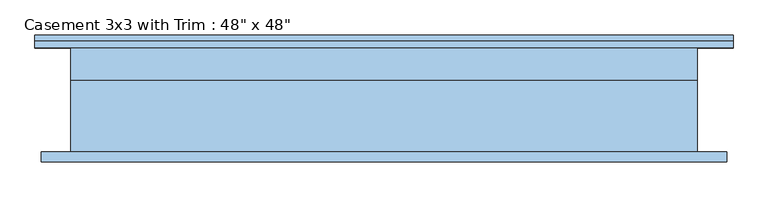
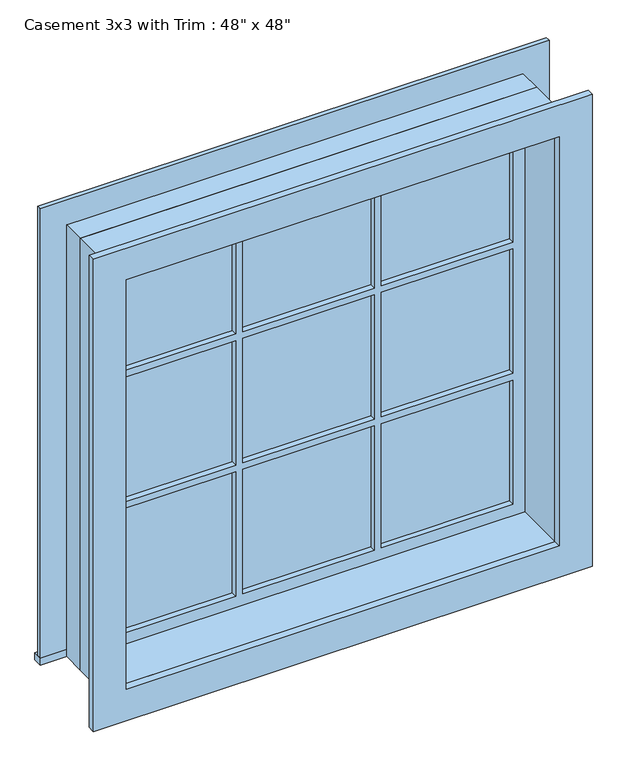
"""IFC4 building model written with IfcOpenShell, lengths in millimetres: window geometry."""

from ifc_helpers import new_model, si_unit, frame, origin, place, context, project, spatial, polyline, outline, extrude, source, transform, mapped, element, save


def window_7418cbd4(model_context):
    return source(origin(), model_context, "Body", "SweptSolid", [
        extrude(outline(polyline([(-679.45, 127.0), (679.45, 127.0), (679.45, 101.6), (-679.45, 101.6), (-679.45, 127.0)])), frame((0.0, 0.0, 914.4), z_axis=(0.0, 0.0, 1.0), x_axis=(1.0, 0.0, 0.0)), (0.0, 0.0, 1.0), 19.05),
        extrude(outline(polyline([(2114.55, -590.55), (2114.55, 590.55), (933.45, 590.55), (933.45, 679.45), (2203.45, 679.45), (2203.45, -679.45), (933.45, -679.45), (933.45, -590.55), (2114.55, -590.55)])), frame((0.0, 101.6, 0.0), z_axis=(0.0, 1.0, 0.0), x_axis=(0.0, 0.0, 1.0)), (0.0, 0.0, 1.0), 12.7),
        extrude(outline(polyline([(194.7333333, 66.675), (546.1, 66.675), (546.1, 53.975), (194.7333333, 53.975), (194.7333333, 66.675)])), frame((0.0, 0.0, 1718.7333333), z_axis=(0.0, 0.0, 1.0), x_axis=(1.0, 0.0, 0.0)), (0.0, 0.0, 1.0), 351.3666667),
        extrude(outline(polyline([(-175.6833333, 66.675), (175.6833333, 66.675), (175.6833333, 53.975), (-175.6833333, 53.975), (-175.6833333, 66.675)])), frame((0.0, 0.0, 1718.7333333), z_axis=(0.0, 0.0, 1.0), x_axis=(1.0, 0.0, 0.0)), (0.0, 0.0, 1.0), 351.3666667),
        extrude(outline(polyline([(-546.1, 66.675), (-194.7333333, 66.675), (-194.7333333, 53.975), (-546.1, 53.975), (-546.1, 66.675)])), frame((0.0, 0.0, 1718.7333333), z_axis=(0.0, 0.0, 1.0), x_axis=(1.0, 0.0, 0.0)), (0.0, 0.0, 1.0), 351.3666667),
        extrude(outline(polyline([(-546.1, 66.675), (-194.7333333, 66.675), (-194.7333333, 53.975), (-546.1, 53.975), (-546.1, 66.675)])), frame((0.0, 0.0, 1348.3166667), z_axis=(0.0, 0.0, 1.0), x_axis=(1.0, 0.0, 0.0)), (0.0, 0.0, 1.0), 351.3666667),
        extrude(outline(polyline([(-175.6833333, 66.675), (175.6833333, 66.675), (175.6833333, 53.975), (-175.6833333, 53.975), (-175.6833333, 66.675)])), frame((0.0, 0.0, 1348.3166667), z_axis=(0.0, 0.0, 1.0), x_axis=(1.0, 0.0, 0.0)), (0.0, 0.0, 1.0), 351.3666667),
        extrude(outline(polyline([(194.7333333, 66.675), (546.1, 66.675), (546.1, 53.975), (194.7333333, 53.975), (194.7333333, 66.675)])), frame((0.0, 0.0, 1348.3166667), z_axis=(0.0, 0.0, 1.0), x_axis=(1.0, 0.0, 0.0)), (0.0, 0.0, 1.0), 351.3666667),
        extrude(outline(polyline([(194.7333333, 66.675), (546.1, 66.675), (546.1, 53.975), (194.7333333, 53.975), (194.7333333, 66.675)])), frame((0.0, 0.0, 977.9), z_axis=(0.0, 0.0, 1.0), x_axis=(1.0, 0.0, 0.0)), (0.0, 0.0, 1.0), 351.3666667),
        extrude(outline(polyline([(-175.6833333, 66.675), (175.6833333, 66.675), (175.6833333, 53.975), (-175.6833333, 53.975), (-175.6833333, 66.675)])), frame((0.0, 0.0, 977.9), z_axis=(0.0, 0.0, 1.0), x_axis=(1.0, 0.0, 0.0)), (0.0, 0.0, 1.0), 351.3666667),
        extrude(outline(polyline([(-546.1, 66.675), (-194.7333333, 66.675), (-194.7333333, 53.975), (-546.1, 53.975), (-546.1, 66.675)])), frame((0.0, 0.0, 977.9), z_axis=(0.0, 0.0, 1.0), x_axis=(1.0, 0.0, 0.0)), (0.0, 0.0, 1.0), 351.3666667),
        extrude(outline(polyline([(2190.75, 666.75), (2190.75, -666.75), (857.25, -666.75), (857.25, 666.75), (2190.75, 666.75)]), holes=[polyline([(2101.85, 577.85), (946.15, 577.85), (946.15, -577.85), (2101.85, -577.85), (2101.85, 577.85)])]), frame((0.0, -120.65, 0.0), z_axis=(0.0, 1.0, 0.0), x_axis=(0.0, 0.0, 1.0)), (0.0, 0.0, 1.0), 19.05),
        extrude(outline(polyline([(2114.55, -590.55), (933.45, -590.55), (933.45, 590.55), (2114.55, 590.55), (2114.55, -590.55)]), holes=[polyline([(2070.1, -194.7333333), (1718.7333333, -194.7333333), (1718.7333333, -546.1), (2070.1, -546.1), (2070.1, -194.7333333)]), polyline([(1699.6833333, -194.7333333), (1348.3166667, -194.7333333), (1348.3166667, -546.1), (1699.6833333, -546.1), (1699.6833333, -194.7333333)]), polyline([(1329.2666667, -194.7333333), (977.9, -194.7333333), (977.9, -546.1), (1329.2666667, -546.1), (1329.2666667, -194.7333333)]), polyline([(2070.1, 175.6833333), (1718.7333333, 175.6833333), (1718.7333333, -175.6833333), (2070.1, -175.6833333), (2070.1, 175.6833333)]), polyline([(1699.6833333, 175.6833333), (1348.3166667, 175.6833333), (1348.3166667, -175.6833333), (1699.6833333, -175.6833333), (1699.6833333, 175.6833333)]), polyline([(1329.2666667, 175.6833333), (977.9, 175.6833333), (977.9, -175.6833333), (1329.2666667, -175.6833333), (1329.2666667, 175.6833333)]), polyline([(2070.1, 546.1), (1718.7333333, 546.1), (1718.7333333, 194.7333333), (2070.1, 194.7333333), (2070.1, 546.1)]), polyline([(1699.6833333, 546.1), (1348.3166667, 546.1), (1348.3166667, 194.7333333), (1699.6833333, 194.7333333), (1699.6833333, 546.1)]), polyline([(1329.2666667, 546.1), (977.9, 546.1), (977.9, 194.7333333), (1329.2666667, 194.7333333), (1329.2666667, 546.1)])]), frame((0.0, 38.1, 0.0), z_axis=(0.0, 1.0, 0.0), x_axis=(0.0, 0.0, 1.0)), (0.0, 0.0, 1.0), 44.45),
        extrude(outline(polyline([(2133.6, -609.6), (914.4, -609.6), (914.4, 609.6), (2133.6, 609.6), (2133.6, -609.6)]), holes=[polyline([(2101.85, -577.85), (2101.85, 577.85), (946.15, 577.85), (946.15, -577.85), (2101.85, -577.85)])]), frame((0.0, -101.6, 0.0), z_axis=(0.0, 1.0, 0.0), x_axis=(0.0, 0.0, 1.0)), (0.0, 0.0, 1.0), 139.7),
        extrude(outline(polyline([(2133.6, 609.6), (2133.6, -609.6), (914.4, -609.6), (914.4, 609.6), (2133.6, 609.6)]), holes=[polyline([(2114.55, 590.55), (933.45, 590.55), (933.45, -590.55), (2114.55, -590.55), (2114.55, 590.55)])]), frame((0.0, 38.1, 0.0), z_axis=(0.0, 1.0, 0.0), x_axis=(0.0, 0.0, 1.0)), (0.0, 0.0, 1.0), 63.5),
    ])


if __name__ == "__main__":
    model = new_model("IFC4")
    model_context = context("Model", 3, world=origin())
    ifc_project = project(units=[si_unit("LENGTHUNIT", "METRE", prefix="MILLI")], contexts=[model_context])
    site = spatial("IfcSite", under=ifc_project)
    building = spatial("IfcBuilding", under=site)
    placement = place(None, origin())
    window_shape = window_7418cbd4(model_context)
    element("IfcWindow", 1, ObjectType="Casement 3x3 with Trim : 48\" x 48\"", at=placement, inside=building, context=model_context, shape_type="MappedRepresentation", body=[
        mapped(window_shape, transform((0.0, 0.0, 0.0), x_axis=(1.0, 0.0, 0.0), y_axis=(0.0, 1.0, 0.0), z_axis=(0.0, 0.0, 1.0))),
    ])
    save(model, "model.ifc")

# Revit data of these elements
# Type "Casement 3x3 with Trim : 48\" x 48\""
#   Type Mark = "10"
#   Construction Type Id = "GSP4R"
#   Assembly Code = "B2020100"
#   Analytic Construction = "1/8 in Pilkington single glazing"
#   Visual Light Transmittance = 0.9
#   Solar Heat Gain Coefficient = 0.78
#   Heat Transfer Coefficient (U) = 0.6496 BTU/(h·ft²·°F)
#   Height = 4' - 0"
#   Default Sill Height = 3' - 0"
#   Trim Projection - Ext. = 0' - 0 1/2"
#   Trim Projection - Int. = 0' - 0 3/4"
#   Trim Width - Exterior = 0' - 3 1/2"
#   Trim Width - Interior = 0' - 3 1/2"
#   Width = 4' - 0"
#   Window Inset = 0' - 0 3/4"
#   Define Thermal Properties by = 1
#   Glass Pane Material = Glass
#   Sash Material = Sash
#   Trim Exterior Material = Trim
#   Trim Interior Material = Trim
#   Wall Closure = (empty or 0)
# Element 1 (IfcWindow, "Casement 3x3 with Trim : 48\" x 48\"")
#   Materials on its faces: "Sash", "Glass", "Trim"
# Materials
#   "Glass": class "Glass", colour RGB 0 128 192, transparency 0.75, Description = "Soda Lime Glass", Cost = 0
#   "Sash": class "Wood", colour RGB 224 178 126, transparency 0
#   "Trim": class "Wood", colour RGB 224 178 126, transparency 0
